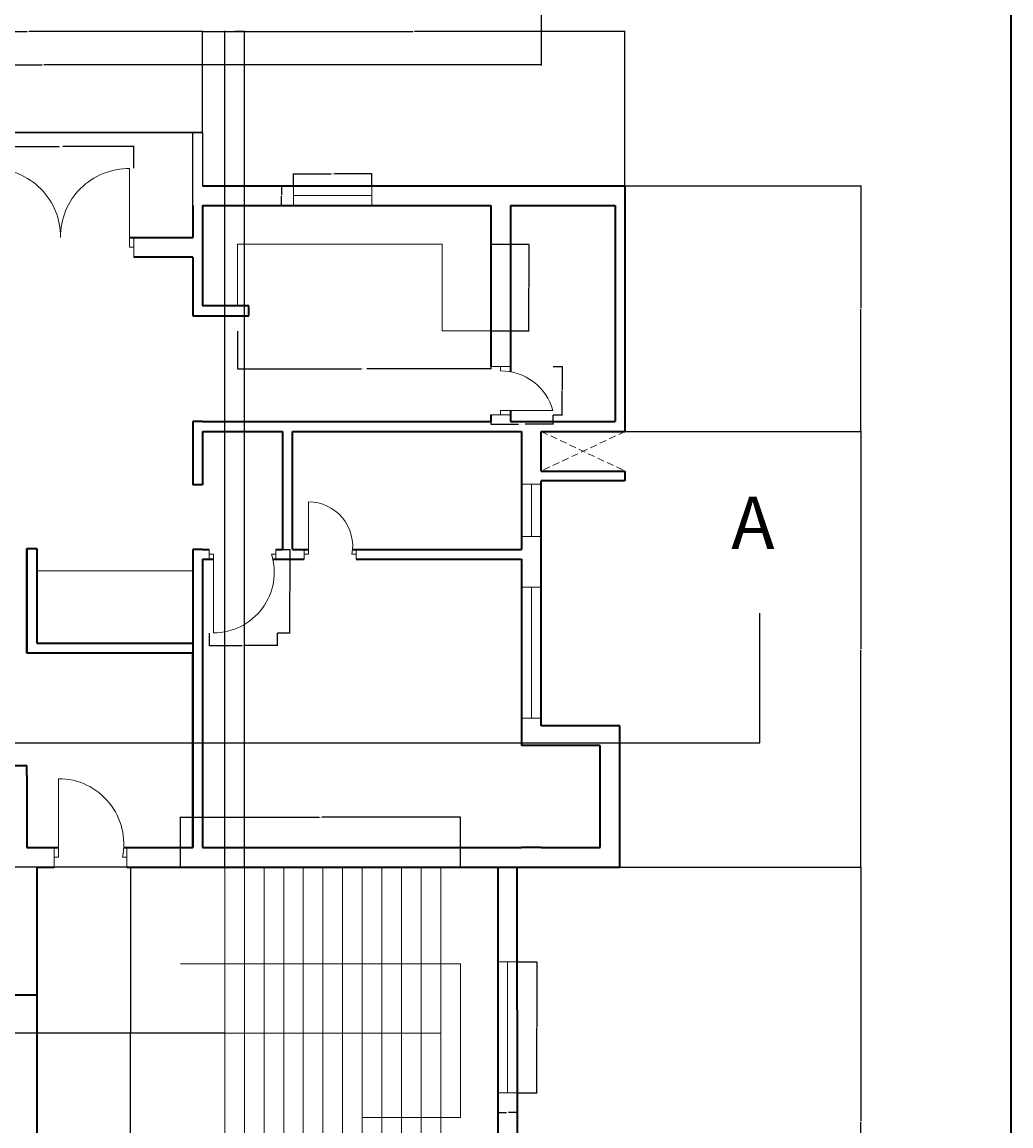
# Model space of a CAD drawing. Units: inches. Extents: x 2296 to 3812, y -1531 to 2564.
# Tile 9 of 10: x 3360 to 3812, y 1720 to 2226. Entities that reach past the tile are written whole.
import ezdxf

# ---------------------------------------------------------------- set-up
doc = ezdxf.new("R2010")
doc.units = ezdxf.units.IN
doc.linetypes.add('HIDDEN2', pattern=[4.7625, 3.175, -1.5875])
for name, color, linetype, lineweight in [('A-ANNO-DIMS', 2, 'Continuous', 18), ('A-ANNO-SYMB', 7, 'Continuous', 25), ('A-ANNO-TTLB', 7, 'Continuous', 35), ('A-DOOR', 3, 'Continuous', 18), ('A-FLOR-CASE', 8, 'Continuous', 18), ('A-FLOR-HRAL', 7, 'Continuous', 25), ('A-FLOR-STRS', 7, 'Continuous', 18), ('A-GLAZ', 4, 'Continuous', 18), ('A-WALL', 7, 'Continuous', 35), ('A-WALL-HIDN', 8, 'HIDDEN2', 18)]:
    doc.layers.add(name, color=color, linetype=linetype, lineweight=lineweight)
doc.styles.get("Standard").update_dxf_attribs({"font": 'arial.ttf'})
doc.dimstyles.get("Standard").update_dxf_attribs({"dimtxt": 0.18, "dimasz": 0.18, "dimexe": 0.18, "dimexo": 0.0625, "dimgap": 0.09, "dimtad": 0, "dimtih": 1, "dimtoh": 1, "dimdec": 4, "dimzin": 0, "dimdsep": 46, "dimtxsty": 'Standard', "dimcen": 0.09, "dimadec": 0, "dimazin": 0, "dimtfac": 1, "dimtdec": 4, "dimtofl": 0, "dimtmove": 0, "dimatfit": 3, "dimfxl": 1, "dimtolj": 1, "dimtzin": 0, "dimarcsym": 0})

# ---------------------------------------------------------------- blocks, each defined once
blk = doc.blocks.new('DOOR-SERVICE-24-NE')
for p, q in [((9, 22.16), (0, 22.16)), ((0, 22.16), (4.5, 22.16)), ((4.5, 22.16), (4.5, 20.16)), ((0, 0), (9, 0)), ((4.5, 0), (4.5, 2)), ((4.5, 2), (28.5, 2)), ((9, 0), (4.5, 0))]:
    blk.add_line(p, q)
blk.add_arc((4.5, -4.78), 24.94, 15.78, 90)
blk = doc.blocks.new('DOOR-BALCONY-PAIR-N')
for p, q in [((2, 4.5), (2, 40.5)), ((64.91, 4.5), (64.91, 40.5)), ((0, 9), (0, 0)), ((66.91, 9), (66.91, 0)), ((0, 0), (0, 4.5)), ((0, 4.5), (2, 4.5)), ((66.91, 4.5), (64.91, 4.5)), ((66.91, 0), (66.91, 4.5))]:
    blk.add_line(p, q)
for centre, radius, start, end in [((2, 9.22), 31.28, 359.5901, 90), ((64.41, 9.36), 31.14, 89.0831, 180.6679)]:
    blk.add_arc(centre, radius, start, end)
blk = doc.blocks.new('DOOR-BEDROOM-36-NE')
for p, q in [((0, 38.25), (0, 33.75)), ((0, 33.75), (0, 36)), ((0, 36), (0, 36)), ((0, 36), (2, 36)), ((2, 36), (2, 0)), ((30.56, 36), (28.56, 36)), ((30.56, 38.25), (30.56, 33.75)), ((30.56, 33.75), (30.56, 36))]:
    blk.add_line(p, q)
blk.add_arc((2, 27.8), 27.8, 270, 17.157)
blk = doc.blocks.new('DOOR-BATH-24-NE')
for p, q in [((2, 2.25), (2, 26.25)), ((0, 4.5), (0, 0)), ((0, 0), (0, 2.25)), ((0, 2.25), (2, 2.25)), ((23.89, 2.25), (21.89, 2.25)), ((23.89, 4.5), (23.89, 0)), ((23.89, 0), (23.89, 2.25))]:
    blk.add_line(p, q)
blk.add_arc((2, 6.01), 20.24, 349.2884, 90)
blk = doc.blocks.new('DOOR-ENTRY-36-N')
for p, q in [((2, 4.5), (2, 40.5)), ((0, 9), (0, 0)), ((33.22, 9), (33.22, 0)), ((0, 0), (0, 4.5)), ((0, 4.5), (2, 4.5)), ((33.22, 4.5), (31.22, 4.5)), ((33.22, 0), (33.22, 4.5))]:
    blk.add_line(p, q)
blk.add_arc((2, 10.64), 29.86, 348.1386, 90)
blk = doc.blocks.new('WIN-36-KITCHEN')
for p, q in [((0, 9), (0, 0)), ((36, 4.5), (36, 9)), ((36, 9), (36, 0)), ((0, 0), (0, 4.5)), ((0, 4.5), (36, 4.5))]:
    blk.add_line(p, q)
blk = doc.blocks.new('WIN-24-BATH')
for p, q in [((4.5, 24), (0, 24)), ((0, 24), (9, 24)), ((4.5, 0), (4.5, 24)), ((0, 0), (9, 0)), ((9, 0), (4.5, 0))]:
    blk.add_line(p, q)
blk = doc.blocks.new('WIN-60-JAMB-A')
for p, q in [((0, 60), (9, 60)), ((9, 60), (4.5, 60)), ((4.5, 60), (4.5, 0)), ((9, 0), (0, 0)), ((4.5, 0), (9, 0))]:
    blk.add_line(p, q)
blk = doc.blocks.new('WIN-60-STAIR')
for p, q in [((0, 59.99), (8.73, 60.01)), ((8.73, 60.01), (4.36, 60)), ((4.36, 60), (4.36, 0)), ((0, 0), (8.81, 0.01)), ((4.36, 0), (0, 0))]:
    blk.add_line(p, q)
blk = doc.blocks.new('STAIR-DOGLEG')
for p, q in [((20.27, 0), (20.27, 152.06)), ((29.27, 0), (29.27, 152.06)), ((38.27, 0), (38.27, 152.06)), ((47.27, 0), (47.27, 152.06)), ((56.27, 0), (56.27, 152.06)), ((65.27, 0), (65.27, 152.06)), ((74.27, 0), (74.27, 152.06)), ((83.27, 0), (83.27, 152.06)), ((92.27, 0), (92.27, 152.06)), ((101.27, 0), (101.27, 152.06)), ((110.27, 0), (110.27, 152.06)), ((119.27, 0), (119.27, 152.06)), ((0, 107.85), (128.27, 107.85)), ((128.27, 107.85), (128.27, 37.4)), ((20.27, 76.03), (119.27, 76.03)), ((128.27, 37.4), (83.27, 37.4))]:
    blk.add_line(p, q)
blk = doc.blocks.new('COUNTER-KITCHEN-N')
for p, q in [((0, 11.4), (0, 39.66)), ((0, 39.66), (93.66, 39.66)), ((93.66, 39.66), (93.66, 0)), ((93.66, 0), (115.91, 0))]:
    blk.add_line(p, q)
blk = doc.blocks.new('*D49')
at = {"layer": 'A-ANNO-DIMS', "color": 0, "lineweight": -2, "transparency": 16777216}
for p, q in [((3431.99, 1838.66), (3409.07, 1838.66)), ((3409.25, 1838.48), (3409.25, 1762.81)), ((3409.25, 1686.78), (3409.25, 1762.45)), ((3431.99, 1686.6), (3409.07, 1686.6))]:
    blk.add_line(p, q, dxfattribs=at)
at = {"layer": 'A-ANNO-DIMS', "color": 0, "transparency": 16777216}
for points in [[(3409.22, 1838.48), (3409.28, 1838.48), (3409.25, 1838.66)], [(3409.22, 1686.78), (3409.28, 1686.78), (3409.25, 1686.6)]]:
    blk.add_solid(points, dxfattribs=at)
at = {"layer": 'Defpoints', "color": 0, "transparency": 16777216}
for p in [(3409.25, 1838.66), (3432.06, 1838.66), (3432.06, 1686.6)]:
    blk.add_point(p, dxfattribs=at)
at = {"layer": 'A-ANNO-DIMS', "color": 0, "transparency": 16777216, "insert": (3409.25, 1762.63), "char_height": 0.18, "attachment_point": 5}
blk.add_mtext('\\A1;STAIR 152 TYP.', dxfattribs=at)
blk = doc.blocks.new('*D50')
at = {"layer": 'A-ANNO-DIMS', "color": 0, "lineweight": -2, "transparency": 16777216}
for p, q in [((3432.06, 1838.72), (3432.06, 1861.65)), ((3432.24, 1861.47), (3495.6, 1861.47)), ((3560.15, 1861.47), (3496.78, 1861.47)), ((3560.33, 1838.72), (3560.33, 1861.65))]:
    blk.add_line(p, q, dxfattribs=at)
at = {"layer": 'A-ANNO-DIMS', "color": 0, "transparency": 16777216}
for points in [[(3432.24, 1861.5), (3432.24, 1861.44), (3432.06, 1861.47)], [(3560.15, 1861.5), (3560.15, 1861.44), (3560.33, 1861.47)]]:
    blk.add_solid(points, dxfattribs=at)
at = {"layer": 'Defpoints', "color": 0, "transparency": 16777216}
for p in [(3560.33, 1861.47), (3432.06, 1838.66), (3560.33, 1838.66)]:
    blk.add_point(p, dxfattribs=at)
at = {"layer": 'A-ANNO-DIMS', "color": 0, "transparency": 16777216, "insert": (3496.19, 1861.47), "char_height": 0.18, "attachment_point": 5}
blk.add_mtext('\\A1;128 TYP.', dxfattribs=at)
blk = doc.blocks.new('*D53')
at = {"layer": 'A-ANNO-DIMS', "color": 0, "lineweight": -2, "transparency": 16777216}
for p, q in [((3458.25, 2084.15), (3458.25, 2066.64)), ((3574.16, 2084.15), (3574.16, 2066.64)), ((3458.43, 2066.82), (3514.95, 2066.82)), ((3573.98, 2066.82), (3517.46, 2066.82))]:
    blk.add_line(p, q, dxfattribs=at)
at = {"layer": 'A-ANNO-DIMS', "color": 0, "transparency": 16777216}
for points in [[(3458.43, 2066.85), (3458.43, 2066.79), (3458.25, 2066.82)], [(3573.98, 2066.85), (3573.98, 2066.79), (3574.16, 2066.82)]]:
    blk.add_solid(points, dxfattribs=at)
at = {"layer": 'Defpoints', "color": 0, "transparency": 16777216}
for p in [(3458.25, 2084.21), (3574.16, 2084.21), (3574.16, 2066.82)]:
    blk.add_point(p, dxfattribs=at)
at = {"layer": 'A-ANNO-DIMS', "color": 0, "transparency": 16777216, "insert": (3516.2, 2066.82), "char_height": 0.18, "attachment_point": 5}
blk.add_mtext('\\A1;COUNTER 116 TYP.', dxfattribs=at)
blk = doc.blocks.new('*D54')
at = {"layer": 'A-ANNO-DIMS', "color": 0, "lineweight": -2, "transparency": 16777216}
for p, q in [((3574.22, 2123.87), (3591.73, 2123.87)), ((3591.55, 2123.69), (3591.55, 2104.22)), ((3591.55, 2084.39), (3591.55, 2103.86)), ((3574.22, 2084.21), (3591.73, 2084.21))]:
    blk.add_line(p, q, dxfattribs=at)
at = {"layer": 'A-ANNO-DIMS', "color": 0, "transparency": 16777216}
for points in [[(3591.52, 2123.69), (3591.58, 2123.69), (3591.55, 2123.87)], [(3591.52, 2084.39), (3591.58, 2084.39), (3591.55, 2084.21)]]:
    blk.add_solid(points, dxfattribs=at)
at = {"layer": 'Defpoints', "color": 0, "transparency": 16777216}
for p in [(3574.16, 2123.87), (3591.55, 2123.87), (3574.16, 2084.21)]:
    blk.add_point(p, dxfattribs=at)
at = {"layer": 'A-ANNO-DIMS', "color": 0, "transparency": 16777216, "insert": (3591.55, 2104.04), "char_height": 0.18, "attachment_point": 5}
blk.add_mtext('\\A1;40 TYP.', dxfattribs=at)
blk = doc.blocks.new('*D61')
at = {"layer": 'A-ANNO-DIMS', "color": 0, "lineweight": -2, "transparency": 16777216}
for p, q in [((3574.16, 2045.69), (3574.16, 2041.3)), ((3602.66, 2045.69), (3602.66, 2041.3)), ((3574.34, 2041.48), (3586.88, 2041.48)), ((3602.48, 2041.48), (3589.94, 2041.48))]:
    blk.add_line(p, q, dxfattribs=at)
at = {"layer": 'A-ANNO-DIMS', "color": 0, "transparency": 16777216}
for points in [[(3574.34, 2041.51), (3574.34, 2041.45), (3574.16, 2041.48)], [(3602.48, 2041.51), (3602.48, 2041.45), (3602.66, 2041.48)]]:
    blk.add_solid(points, dxfattribs=at)
at = {"layer": 'Defpoints', "color": 0, "transparency": 16777216}
for p in [(3574.16, 2045.75), (3602.66, 2045.75), (3602.66, 2041.48)]:
    blk.add_point(p, dxfattribs=at)
at = {"layer": 'A-ANNO-DIMS', "color": 0, "transparency": 16777216, "insert": (3588.41, 2041.48), "char_height": 0.18, "attachment_point": 5}
blk.add_mtext('\\A1;SERVICE DOOR 29 TYP.', dxfattribs=at)
blk = doc.blocks.new('*D62')
at = {"layer": 'A-ANNO-DIMS', "color": 0, "lineweight": -2, "transparency": 16777216}
for p, q in [((3602.72, 2067.91), (3607.11, 2067.91)), ((3606.93, 2067.73), (3606.93, 2057.01)), ((3606.93, 2045.93), (3606.93, 2056.65)), ((3602.72, 2045.75), (3607.11, 2045.75))]:
    blk.add_line(p, q, dxfattribs=at)
at = {"layer": 'A-ANNO-DIMS', "color": 0, "transparency": 16777216}
for points in [[(3606.9, 2067.73), (3606.96, 2067.73), (3606.93, 2067.91)], [(3606.9, 2045.93), (3606.96, 2045.93), (3606.93, 2045.75)]]:
    blk.add_solid(points, dxfattribs=at)
at = {"layer": 'Defpoints', "color": 0, "transparency": 16777216}
for p in [(3602.66, 2067.91), (3606.93, 2067.91), (3602.66, 2045.75)]:
    blk.add_point(p, dxfattribs=at)
at = {"layer": 'A-ANNO-DIMS', "color": 0, "transparency": 16777216, "insert": (3606.93, 2056.83), "char_height": 0.18, "attachment_point": 5}
blk.add_mtext('\\A1;22 TYP.', dxfattribs=at)
blk = doc.blocks.new('*D63')
at = {"layer": 'A-ANNO-DIMS', "color": 0, "lineweight": -2, "transparency": 16777216}
for p, q in [((3343.86, 2158.72), (3343.86, 2168.88)), ((3344.04, 2168.7), (3376.46, 2168.7)), ((3410.59, 2168.7), (3378.17, 2168.7)), ((3410.77, 2158.72), (3410.77, 2168.88))]:
    blk.add_line(p, q, dxfattribs=at)
at = {"layer": 'A-ANNO-DIMS', "color": 0, "transparency": 16777216}
for points in [[(3344.04, 2168.73), (3344.04, 2168.67), (3343.86, 2168.7)], [(3410.59, 2168.73), (3410.59, 2168.67), (3410.77, 2168.7)]]:
    blk.add_solid(points, dxfattribs=at)
at = {"layer": 'Defpoints', "color": 0, "transparency": 16777216}
for p in [(3410.77, 2168.7), (3343.86, 2158.66), (3410.77, 2158.66)]:
    blk.add_point(p, dxfattribs=at)
at = {"layer": 'A-ANNO-DIMS', "color": 0, "transparency": 16777216, "insert": (3377.32, 2168.7), "char_height": 0.18, "attachment_point": 5}
blk.add_mtext('\\A1;PAIR 67 TYP.', dxfattribs=at)
blk = doc.blocks.new('*D65')
at = {"layer": 'A-ANNO-DIMS', "color": 0, "lineweight": -2, "transparency": 16777216}
for p, q in [((3476.44, 1984.16), (3482.29, 1984.16)), ((3482.11, 1983.98), (3482.11, 1965.22)), ((3482.11, 1946.09), (3482.11, 1964.85)), ((3476.44, 1945.91), (3482.29, 1945.91))]:
    blk.add_line(p, q, dxfattribs=at)
at = {"layer": 'A-ANNO-DIMS', "color": 0, "transparency": 16777216}
for points in [[(3482.08, 1983.98), (3482.14, 1983.98), (3482.11, 1984.16)], [(3482.08, 1946.09), (3482.14, 1946.09), (3482.11, 1945.91)]]:
    blk.add_solid(points, dxfattribs=at)
at = {"layer": 'Defpoints', "color": 0, "transparency": 16777216}
for p in [(3476.37, 1984.16), (3482.11, 1984.16), (3476.37, 1945.91)]:
    blk.add_point(p, dxfattribs=at)
at = {"layer": 'A-ANNO-DIMS', "color": 0, "transparency": 16777216, "insert": (3482.11, 1965.03), "char_height": 0.18, "attachment_point": 5}
blk.add_mtext('\\A1;DOOR 38 TYP.', dxfattribs=at)
blk = doc.blocks.new('*D66')
at = {"layer": 'A-ANNO-DIMS', "color": 0, "lineweight": -2, "transparency": 16777216}
for p, q in [((3445.21, 1945.85), (3445.21, 1939.99)), ((3476.37, 1945.85), (3476.37, 1939.99)), ((3445.39, 1940.17), (3460.26, 1940.17)), ((3476.19, 1940.17), (3461.32, 1940.17))]:
    blk.add_line(p, q, dxfattribs=at)
at = {"layer": 'A-ANNO-DIMS', "color": 0, "transparency": 16777216}
for points in [[(3445.39, 1940.2), (3445.39, 1940.14), (3445.21, 1940.17)], [(3476.19, 1940.2), (3476.19, 1940.14), (3476.37, 1940.17)]]:
    blk.add_solid(points, dxfattribs=at)
at = {"layer": 'Defpoints', "color": 0, "transparency": 16777216}
for p in [(3445.21, 1945.91), (3476.37, 1945.91), (3476.37, 1940.17)]:
    blk.add_point(p, dxfattribs=at)
at = {"layer": 'A-ANNO-DIMS', "color": 0, "transparency": 16777216, "insert": (3460.79, 1940.17), "char_height": 0.18, "attachment_point": 5}
blk.add_mtext('\\A1;31 TYP.', dxfattribs=at)
blk = doc.blocks.new('*D99')
at = {"layer": 'A-ANNO-DIMS', "color": 0, "lineweight": -2, "transparency": 16777216}
for p, q in [((3483.78, 2150.72), (3483.78, 2156.24)), ((3483.96, 2156.06), (3500.94, 2156.06)), ((3519.6, 2156.06), (3502.63, 2156.06)), ((3519.78, 2150.72), (3519.78, 2156.24))]:
    blk.add_line(p, q, dxfattribs=at)
at = {"layer": 'A-ANNO-DIMS', "color": 0, "transparency": 16777216}
for points in [[(3483.96, 2156.09), (3483.96, 2156.03), (3483.78, 2156.06)], [(3519.6, 2156.09), (3519.6, 2156.03), (3519.78, 2156.06)]]:
    blk.add_solid(points, dxfattribs=at)
at = {"layer": 'Defpoints', "color": 0, "transparency": 16777216}
for p in [(3519.78, 2156.06), (3483.78, 2150.66), (3519.78, 2150.66)]:
    blk.add_point(p, dxfattribs=at)
at = {"layer": 'A-ANNO-DIMS', "color": 0, "transparency": 16777216, "insert": (3501.78, 2156.06), "char_height": 0.18, "attachment_point": 5}
blk.add_mtext('\\A1;WIN. 36 TYP.', dxfattribs=at)
blk = doc.blocks.new('*D100')
at = {"layer": 'A-ANNO-DIMS', "color": 0, "lineweight": -2, "transparency": 16777216}
for p, q in [((3483.72, 2150.66), (3478.2, 2150.66)), ((3478.38, 2150.48), (3478.38, 2146.34)), ((3478.38, 2141.84), (3478.38, 2145.98)), ((3483.72, 2141.66), (3478.2, 2141.66))]:
    blk.add_line(p, q, dxfattribs=at)
at = {"layer": 'A-ANNO-DIMS', "color": 0, "transparency": 16777216}
for points in [[(3478.35, 2150.48), (3478.41, 2150.48), (3478.38, 2150.66)], [(3478.35, 2141.84), (3478.41, 2141.84), (3478.38, 2141.66)]]:
    blk.add_solid(points, dxfattribs=at)
at = {"layer": 'Defpoints', "color": 0, "transparency": 16777216}
for p in [(3478.38, 2150.66), (3483.78, 2150.66), (3483.78, 2141.66)]:
    blk.add_point(p, dxfattribs=at)
at = {"layer": 'A-ANNO-DIMS', "color": 0, "transparency": 16777216, "insert": (3478.38, 2146.16), "char_height": 0.18, "attachment_point": 5}
blk.add_mtext('\\A1;9 TYP.', dxfattribs=at)
blk = doc.blocks.new('*D113')
at = {"layer": 'A-ANNO-DIMS', "color": 0, "lineweight": -2, "transparency": 16777216}
for p, q in [((3586.37, 1795.35), (3595.49, 1795.35)), ((3595.31, 1795.17), (3595.31, 1765.53)), ((3595.31, 1735.52), (3595.31, 1765.16)), ((3586.37, 1735.34), (3595.49, 1735.34))]:
    blk.add_line(p, q, dxfattribs=at)
at = {"layer": 'A-ANNO-DIMS', "color": 0, "transparency": 16777216}
for points in [[(3595.28, 1795.17), (3595.34, 1795.17), (3595.31, 1795.35)], [(3595.28, 1735.52), (3595.34, 1735.52), (3595.31, 1735.34)]]:
    blk.add_solid(points, dxfattribs=at)
at = {"layer": 'Defpoints', "color": 0, "transparency": 16777216}
for p in [(3586.31, 1795.35), (3595.31, 1795.35), (3586.31, 1735.34)]:
    blk.add_point(p, dxfattribs=at)
at = {"layer": 'A-ANNO-DIMS', "color": 0, "transparency": 16777216, "insert": (3595.31, 1765.34), "char_height": 0.18, "attachment_point": 5}
blk.add_mtext('\\A1;WINDOW 60 TYP.', dxfattribs=at)
blk = doc.blocks.new('*D114')
at = {"layer": 'A-ANNO-DIMS', "color": 0, "lineweight": -2, "transparency": 16777216}
for p, q in [((3577.49, 1735.28), (3577.49, 1726.16)), ((3586.31, 1735.28), (3586.31, 1726.16)), ((3577.67, 1726.34), (3581.44, 1726.34)), ((3586.13, 1726.34), (3582.36, 1726.34))]:
    blk.add_line(p, q, dxfattribs=at)
at = {"layer": 'A-ANNO-DIMS', "color": 0, "transparency": 16777216}
for points in [[(3577.67, 1726.37), (3577.67, 1726.31), (3577.49, 1726.34)], [(3586.13, 1726.37), (3586.13, 1726.31), (3586.31, 1726.34)]]:
    blk.add_solid(points, dxfattribs=at)
at = {"layer": 'Defpoints', "color": 0, "transparency": 16777216}
for p in [(3577.49, 1735.34), (3586.31, 1735.34), (3586.31, 1726.34)]:
    blk.add_point(p, dxfattribs=at)
at = {"layer": 'A-ANNO-DIMS', "color": 0, "transparency": 16777216, "insert": (3581.9, 1726.34), "char_height": 0.18, "attachment_point": 5}
blk.add_mtext('\\A1;9 TYP.', dxfattribs=at)
blk = doc.blocks.new('*D132')
at = {"layer": 'A-ANNO-DIMS', "color": 0, "lineweight": -2, "transparency": 16777216}
for p, q in [((3282.51, 2175.09), (3282.51, 2221.56)), ((3282.69, 2221.38), (3361.88, 2221.38)), ((3441.98, 2221.38), (3362.79, 2221.38)), ((3442.16, 2175.09), (3442.16, 2221.56))]:
    blk.add_line(p, q, dxfattribs=at)
at = {"layer": 'A-ANNO-DIMS', "color": 0, "transparency": 16777216}
for points in [[(3282.69, 2221.41), (3282.69, 2221.35), (3282.51, 2221.38)], [(3441.98, 2221.41), (3441.98, 2221.35), (3442.16, 2221.38)]]:
    blk.add_solid(points, dxfattribs=at)
at = {"layer": 'Defpoints', "color": 0, "transparency": 16777216}
for p in [(3442.16, 2221.38), (3282.51, 2175.03), (3442.16, 2175.03)]:
    blk.add_point(p, dxfattribs=at)
at = {"layer": 'A-ANNO-DIMS', "color": 0, "transparency": 16777216, "insert": (3362.33, 2221.38), "char_height": 0.18, "attachment_point": 5}
blk.add_mtext('\\A1;159.65', dxfattribs=at)
blk = doc.blocks.new('*D133')
at = {"layer": 'A-ANNO-DIMS', "color": 0, "lineweight": -2, "transparency": 16777216}
for p, q in [((3442.16, 2175.09), (3442.16, 2221.56)), ((3442.34, 2221.38), (3538.52, 2221.38)), ((3635.48, 2221.38), (3539.29, 2221.38)), ((3635.66, 2150.72), (3635.66, 2221.56))]:
    blk.add_line(p, q, dxfattribs=at)
at = {"layer": 'A-ANNO-DIMS', "color": 0, "transparency": 16777216}
for points in [[(3442.34, 2221.41), (3442.34, 2221.35), (3442.16, 2221.38)], [(3635.48, 2221.41), (3635.48, 2221.35), (3635.66, 2221.38)]]:
    blk.add_solid(points, dxfattribs=at)
at = {"layer": 'Defpoints', "color": 0, "transparency": 16777216}
for p in [(3635.66, 2221.38), (3442.16, 2175.03), (3635.66, 2150.66)]:
    blk.add_point(p, dxfattribs=at)
at = {"layer": 'A-ANNO-DIMS', "color": 0, "transparency": 16777216, "insert": (3538.91, 2221.38), "char_height": 0.18, "attachment_point": 5}
blk.add_mtext('\\A1;193.5', dxfattribs=at)
blk = doc.blocks.new('*D136')
at = {"layer": 'A-ANNO-DIMS', "color": 0, "lineweight": -2, "transparency": 16777216}
for p, q in [((3633.38, 1838.66), (3743.91, 1838.66)), ((3743.73, 1838.48), (3743.73, 1722.31)), ((3743.73, 1605.78), (3743.73, 1721.95)), ((3642.06, 1605.6), (3743.91, 1605.6))]:
    blk.add_line(p, q, dxfattribs=at)
at = {"layer": 'A-ANNO-DIMS', "color": 0, "transparency": 16777216}
for points in [[(3743.7, 1838.48), (3743.76, 1838.48), (3743.73, 1838.66)], [(3743.7, 1605.78), (3743.76, 1605.78), (3743.73, 1605.6)]]:
    blk.add_solid(points, dxfattribs=at)
at = {"layer": 'Defpoints', "color": 0, "transparency": 16777216}
for p in [(3633.32, 1838.66), (3743.73, 1838.66), (3641.99, 1605.6)]:
    blk.add_point(p, dxfattribs=at)
at = {"layer": 'A-ANNO-DIMS', "color": 0, "transparency": 16777216, "insert": (3743.73, 1722.13), "char_height": 0.18, "attachment_point": 5}
blk.add_mtext('\\A1;233.06', dxfattribs=at)
blk = doc.blocks.new('*D137')
at = {"layer": 'A-ANNO-DIMS', "color": 0, "lineweight": -2, "transparency": 16777216}
for p, q in [((3635.72, 2038.16), (3743.91, 2038.16)), ((3743.73, 2037.98), (3743.73, 1938.59)), ((3743.73, 1838.84), (3743.73, 1938.23)), ((3633.38, 1838.66), (3743.91, 1838.66))]:
    blk.add_line(p, q, dxfattribs=at)
at = {"layer": 'A-ANNO-DIMS', "color": 0, "transparency": 16777216}
for points in [[(3743.7, 2037.98), (3743.76, 2037.98), (3743.73, 2038.16)], [(3743.7, 1838.84), (3743.76, 1838.84), (3743.73, 1838.66)]]:
    blk.add_solid(points, dxfattribs=at)
at = {"layer": 'Defpoints', "color": 0, "transparency": 16777216}
for p in [(3635.66, 2038.16), (3743.73, 2038.16), (3633.32, 1838.66)]:
    blk.add_point(p, dxfattribs=at)
at = {"layer": 'A-ANNO-DIMS', "color": 0, "transparency": 16777216, "insert": (3743.73, 1938.41), "char_height": 0.18, "attachment_point": 5}
blk.add_mtext('\\A1;199.5', dxfattribs=at)
blk = doc.blocks.new('*D138')
at = {"layer": 'A-ANNO-DIMS', "color": 0, "lineweight": -2, "transparency": 16777216}
for p, q in [((3635.72, 2150.66), (3743.91, 2150.66)), ((3743.73, 2150.48), (3743.73, 2094.59)), ((3743.73, 2038.34), (3743.73, 2094.23)), ((3635.72, 2038.16), (3743.91, 2038.16))]:
    blk.add_line(p, q, dxfattribs=at)
at = {"layer": 'A-ANNO-DIMS', "color": 0, "transparency": 16777216}
for points in [[(3743.7, 2150.48), (3743.76, 2150.48), (3743.73, 2150.66)], [(3743.7, 2038.34), (3743.76, 2038.34), (3743.73, 2038.16)]]:
    blk.add_solid(points, dxfattribs=at)
at = {"layer": 'Defpoints', "color": 0, "transparency": 16777216}
for p in [(3635.66, 2150.66), (3743.73, 2150.66), (3635.66, 2038.16)]:
    blk.add_point(p, dxfattribs=at)
at = {"layer": 'A-ANNO-DIMS', "color": 0, "transparency": 16777216, "insert": (3743.73, 2094.41), "char_height": 0.18, "attachment_point": 5}
blk.add_mtext('\\A1;112.5', dxfattribs=at)
blk = doc.blocks.new('*D140')
at = {"layer": 'A-ANNO-DIMS', "color": 0, "lineweight": -2, "transparency": 16777216}
for p, q in [((3452.33, 1838.72), (3452.33, 2221.56)), ((3452.51, 2221.38), (3456.68, 2221.38)), ((3461.15, 2221.38), (3456.98, 2221.38)), ((3461.33, 1838.72), (3461.33, 2221.56))]:
    blk.add_line(p, q, dxfattribs=at)
at = {"layer": 'A-ANNO-DIMS', "color": 0, "transparency": 16777216}
for points in [[(3452.51, 2221.41), (3452.51, 2221.35), (3452.33, 2221.38)], [(3461.15, 2221.41), (3461.15, 2221.35), (3461.33, 2221.38)]]:
    blk.add_solid(points, dxfattribs=at)
at = {"layer": 'Defpoints', "color": 0, "transparency": 16777216}
for p in [(3461.33, 2221.38), (3452.33, 1838.66), (3461.33, 1838.66)]:
    blk.add_point(p, dxfattribs=at)
at = {"layer": 'A-ANNO-DIMS', "color": 0, "transparency": 16777216, "insert": (3456.83, 2221.38), "char_height": 0.18, "attachment_point": 5}
blk.add_mtext('\\A1;9', dxfattribs=at)
blk = doc.blocks.new('*D141')
at = {"layer": 'A-ANNO-DIMS', "color": 0, "lineweight": -2, "transparency": 16777216}
for p, q in [((3452.27, 1838.66), (3014.48, 1838.66)), ((3014.66, 1838.48), (3014.66, 1800.83)), ((3014.66, 1762.81), (3014.66, 1800.46)), ((3452.27, 1762.63), (3014.48, 1762.63))]:
    blk.add_line(p, q, dxfattribs=at)
at = {"layer": 'A-ANNO-DIMS', "color": 0, "transparency": 16777216}
for points in [[(3014.63, 1838.48), (3014.69, 1838.48), (3014.66, 1838.66)], [(3014.63, 1762.81), (3014.69, 1762.81), (3014.66, 1762.63)]]:
    blk.add_solid(points, dxfattribs=at)
at = {"layer": 'Defpoints', "color": 0, "transparency": 16777216}
for p in [(3014.66, 1838.66), (3452.33, 1838.66), (3452.33, 1762.63)]:
    blk.add_point(p, dxfattribs=at)
at = {"layer": 'A-ANNO-DIMS', "color": 0, "transparency": 16777216, "insert": (3014.66, 1800.64), "char_height": 0.18, "attachment_point": 5}
blk.add_mtext('\\A1;76.03', dxfattribs=at)
blk = doc.blocks.new('*D159')
at = {"layer": 'A-ANNO-DIMS', "color": 0, "lineweight": -2, "transparency": 16777216}
for p, q in [((3140.84, 2277.72), (3140.84, 2205.81)), ((3597.32, 2277.72), (3597.32, 2205.81)), ((3141.02, 2205.99), (3368.68, 2205.99)), ((3597.14, 2205.99), (3369.48, 2205.99))]:
    blk.add_line(p, q, dxfattribs=at)
at = {"layer": 'A-ANNO-DIMS', "color": 0, "transparency": 16777216}
for points in [[(3141.02, 2206.02), (3141.02, 2205.96), (3140.84, 2205.99)], [(3597.14, 2206.02), (3597.14, 2205.96), (3597.32, 2205.99)]]:
    blk.add_solid(points, dxfattribs=at)
at = {"layer": 'Defpoints', "color": 0, "transparency": 16777216}
for p in [(3140.84, 2277.78), (3597.32, 2277.78), (3597.32, 2205.99)]:
    blk.add_point(p, dxfattribs=at)
at = {"layer": 'A-ANNO-DIMS', "color": 0, "transparency": 16777216, "insert": (3369.08, 2205.99), "char_height": 0.18, "attachment_point": 5}
blk.add_mtext('\\A1;456.5', dxfattribs=at)

msp = doc.modelspace()

# ---------------------------------------------------------------- linework, layer by layer
at = {"layer": 'A-ANNO-SYMB'}
for p, q in [((3697.3821, 1895.5359), (3697.3821, 1954.9583)), ((3061.0144, 1895.5359), (3697.3821, 1895.5359))]:
    msp.add_line(p, q, dxfattribs=at)
at = {"layer": 'A-ANNO-TTLB'}
msp.add_lwpolyline([(2296.1257, 2564.2989), (3812.4193, 2564.2989), (3812.4193, 1124.0028), (2296.1257, 1124.0028)], close=True, dxfattribs=at)
at = {"layer": 'A-FLOR-CASE'}
msp.add_line((3437.6588, 1974.3293), (3366.2648, 1974.3293), dxfattribs=at)
at = {"layer": 'A-FLOR-HRAL'}
for p, q in [((3442.1588, 2175.0276), (3308.6588, 2175.0276)), ((3313.1588, 2175.0276), (3442.1588, 2175.0276)), ((3437.6588, 2141.6578), (3437.6588, 2175.0276)), ((3442.1588, 2175.0276), (3442.1588, 2150.6578))]:
    msp.add_line(p, q, dxfattribs=at)
at = {"layer": 'A-WALL'}
for p, q in [((3442.1588, 2150.6578), (3635.6588, 2150.6578)), ((3442.1588, 2150.6578), (3635.6588, 2150.6578)), ((3635.6588, 2150.6578), (3635.6588, 2038.1578)), ((3437.6588, 2141.6578), (3437.6588, 2127.0276)), ((3442.1588, 2141.6578), (3442.1588, 2095.613)), ((3442.1588, 2141.6578), (3574.1588, 2141.6578)), ((3574.1588, 2141.6578), (3574.1588, 2067.9121)), ((3583.1588, 2141.6578), (3583.1588, 2065.5027)), ((3583.1588, 2141.6578), (3631.1588, 2141.6578)), ((3631.1588, 2141.6578), (3631.1588, 2042.6578)), ((3408.7726, 2127.0276), (3437.6588, 2127.0276)), ((3437.6588, 2118.0276), (3410.7726, 2118.0276)), ((3437.6588, 2118.0276), (3437.6588, 2091.113)), ((3463.3407, 2095.613), (3442.1588, 2095.613)), ((3463.3407, 2091.113), (3463.3407, 2095.613)), ((3437.6588, 2091.113), (3463.3407, 2091.113)), ((3583.1588, 2047.7544), (3583.1588, 2042.6578)), ((3437.6588, 2042.6578), (3437.6588, 2013.7336)), ((3442.1588, 2042.6578), (3437.6588, 2042.6578)), ((3442.1588, 2042.6578), (3574.1588, 2042.6578)), ((3574.1588, 2045.7544), (3574.1588, 2042.6578)), ((3583.1588, 2042.6578), (3631.1588, 2042.6578)), ((3583.1588, 2042.6578), (3631.1588, 2042.6578)), ((3442.1588, 2038.1578), (3442.1588, 2013.7336)), ((3442.1588, 2038.1578), (3478.8177, 2038.1578)), ((3478.8177, 2038.1578), (3478.8177, 1984.1578)), ((3483.3177, 2038.1578), (3588.3177, 2038.1578)), ((3483.3177, 1984.1578), (3483.3177, 2038.1578)), ((3483.3177, 2038.1578), (3588.3177, 2038.1578)), ((3588.3177, 2038.1578), (3588.3177, 1984.1578)), ((3597.3177, 2038.1578), (3635.6588, 2038.1578)), ((3597.3177, 2020.0533), (3597.3177, 2038.1578)), ((3597.3177, 2020.0533), (3635.6588, 2020.0533)), ((3635.6588, 2020.0533), (3635.6588, 2015.5533)), ((3635.6588, 2020.0533), (3635.6588, 2015.5533)), ((3442.1588, 2013.7336), (3437.6588, 2013.7336)), ((3597.3177, 1990.1003), (3597.3177, 2015.5533)), ((3635.6588, 2015.5533), (3597.3177, 2015.5533)), ((3597.3177, 2011.1578), (3597.3177, 2011.1578)), ((3597.3177, 1984.1578), (3597.3177, 2006.6578)), ((3361.7648, 1984.5954), (3361.7648, 1936.6578)), ((3361.7648, 1936.6578), (3361.7648, 1984.5954)), ((3361.7648, 1984.5954), (3366.2648, 1984.5954)), ((3366.2648, 1984.5954), (3366.2648, 1941.1578)), ((3437.6588, 1984.1578), (3437.6588, 1847.6578)), ((3442.1588, 1984.1578), (3437.6588, 1984.1578)), ((3437.6588, 1984.1578), (3437.6588, 1979.704)), ((3442.1588, 1984.1578), (3445.2067, 1984.1578)), ((3475.769, 1984.1578), (3478.8177, 1984.1578)), ((3483.3177, 1984.1578), (3490.7043, 1984.1578)), ((3510.8861, 1984.1578), (3588.3177, 1984.1578)), ((3597.3177, 1903.3996), (3597.3177, 1984.1578)), ((3442.1588, 1979.6578), (3442.1588, 1847.6578)), ((3442.1588, 1979.6578), (3447.2067, 1979.6578)), ((3474.3618, 1979.6578), (3488.7043, 1979.6578)), ((3512.59, 1979.6578), (3588.3177, 1979.6578)), ((3588.3177, 1979.6578), (3588.3177, 1894.3996)), ((3366.2648, 1941.1578), (3437.6588, 1941.1578)), ((3437.6588, 1936.6578), (3361.7648, 1936.6578)), ((3437.6588, 1847.6578), (3437.6588, 1936.6578)), ((3633.3177, 1903.3996), (3597.3177, 1903.3996)), ((3633.3177, 1894.3996), (3633.3177, 1903.3996)), ((3597.3177, 1894.3996), (3588.3177, 1894.3996)), ((3624.3177, 1894.3996), (3597.3177, 1894.3996)), ((3624.3177, 1847.6578), (3624.3177, 1894.3996)), ((3633.3177, 1838.6578), (3633.3177, 1894.3996)), ((3277.1479, 1885.1578), (3361.7648, 1885.1578)), ((3361.7648, 1880.6578), (3361.7648, 1885.1578)), ((3361.7648, 1880.6578), (3361.7648, 1847.6578)), ((3361.7648, 1847.6578), (3366.2648, 1847.6578)), ((3366.2648, 1847.6578), (3376.2592, 1847.6578)), ((3366.2648, 1847.6578), (3376.2592, 1847.6578)), ((3406.0762, 1847.6578), (3437.6588, 1847.6578)), ((3406.0762, 1847.6578), (3437.6588, 1847.6578)), ((3442.1588, 1847.6578), (3588.3177, 1847.6578)), ((3442.1588, 1847.6578), (3588.3177, 1847.6578)), ((3597.3177, 1847.6578), (3588.3177, 1847.6578)), ((3597.3177, 1847.6578), (3612.3177, 1847.6578)), ((3612.3177, 1847.6578), (3624.3177, 1847.6578)), ((3366.2648, 1838.6578), (3374.2592, 1838.6578)), ((3366.2648, 1838.6578), (3366.2648, 1780.1578)), ((3366.2648, 1838.6578), (3366.2648, 1789.1578)), ((3407.4836, 1838.6578), (3442.1588, 1838.6578)), ((3442.1588, 1838.6578), (3597.3177, 1838.6578)), ((3442.1588, 1838.6578), (3586.1588, 1838.6578)), ((3577.4944, 1686.6012), (3577.4944, 1838.6578)), ((3586.1588, 1838.6578), (3586.4944, 1605.6012)), ((3588.3177, 1838.6578), (3597.3177, 1838.6578)), ((3597.3177, 1838.6578), (3624.3177, 1838.6578)), ((3624.3177, 1838.6578), (3633.3177, 1838.6578)), ((3291.4894, 1780.1578), (3366.2648, 1780.1578)), ((3366.2648, 1780.1578), (3366.2648, 1674.9485))]:
    msp.add_line(p, q, dxfattribs=at)
at = {"layer": 'A-WALL-HIDN'}
for p, q in [((3635.6588, 2038.1578), (3597.3177, 2020.0533)), ((3597.3177, 2038.1578), (3635.6588, 2020.0533)), ((3635.6588, 2020.0533), (3635.6588, 2020.0533))]:
    msp.add_line(p, q, dxfattribs=at)

# ---------------------------------------------------------------- block references
at = {"layer": 'A-DOOR'}
for name, p in [('DOOR-BALCONY-PAIR-N', (3343.8604, 2118.028)), ('DOOR-SERVICE-24-NE', (3574.1584, 2045.754)), ('DOOR-BATH-24-NE', (3488.7044, 1979.658)), ('DOOR-BEDROOM-36-NE', (3445.2064, 1945.908)), ('DOOR-ENTRY-36-N', (3374.2594, 1838.658))]:
    msp.add_blockref(name, p, dxfattribs=at)
at = {"layer": 'A-FLOR-CASE'}
msp.add_blockref('COUNTER-KITCHEN-N', (3458.2474, 2084.209), dxfattribs=at)
at = {"layer": 'A-FLOR-STRS'}
msp.add_blockref('STAIR-DOGLEG', (3432.0574, 1686.601), dxfattribs=at)
at = {"layer": 'A-GLAZ'}
for name, p in [('WIN-36-KITCHEN', (3483.7844, 2141.658)), ('WIN-24-BATH', (3588.3174, 1990.1)), ('WIN-60-JAMB-A', (3588.3174, 1906.83)), ('WIN-60-STAIR', (3577.4944, 1735.339))]:
    msp.add_blockref(name, p, dxfattribs=at)

# ---------------------------------------------------------------- texts
at = {"layer": 'A-ANNO-SYMB', "insert": (3684.287, 2008.2679), "char_height": 24, "attachment_point": 1}
msp.add_mtext_dynamic_manual_height_columns('A', width=30.195569, gutter_width=12.5, heights=[0], dxfattribs=at)

# ---------------------------------------------------------------- dimensions: what is measured, and where the dimension line sits
at = {"layer": 'A-ANNO-DIMS'}
for base, p1, p2, override, picture, middle in [((3597.3177, 2205.9928), (3140.8418, 2277.7848), (3597.3177, 2277.7848), {"dimdec": 1, "dimlfac": 1, "dimrnd": 0, "dimzin": 0, "dimdsep": 46, "dimlunit": 2}, '*D159', (3369.0797, 2205.9928)), ((3442.1588, 2221.3776), (3282.5073, 2175.0276), (3442.1588, 2175.0276), {"dimdec": 2, "dimlfac": 1, "dimrnd": 0, "dimzin": 0, "dimdsep": 46, "dimlunit": 2}, '*D132', (3362.333, 2221.3776)), ((3635.6588, 2221.3776), (3442.1588, 2175.0276), (3635.6588, 2150.6578), {"dimdec": 1, "dimlfac": 1, "dimrnd": 0, "dimzin": 0, "dimdsep": 46, "dimlunit": 2}, '*D133', (3538.9088, 2221.3776)), ((3461.3277, 2221.3776), (3452.3277, 1838.6578), (3461.3277, 1838.6578), {"dimdec": 0, "dimlfac": 1, "dimrnd": 0, "dimzin": 0, "dimdsep": 46, "dimlunit": 2}, '*D140', (3456.8277, 2221.3776))]:
    dim = msp.add_linear_dim(base=base, p1=p1, p2=p2, dimstyle='Standard', override=override, dxfattribs=at)
    dim.commit()
    dim.dimension.update_dxf_attribs({"geometry": picture, "text_midpoint": middle})
for base, p1, p2, text, picture, middle in [((3410.7726, 2168.699), (3343.86, 2158.6621), (3410.7726, 2158.6621), 'PAIR <> TYP.', '*D63', (3377.3163, 2168.699)), ((3519.7848, 2156.0578), (3483.7848, 2150.6578), (3519.7848, 2150.6578), 'WIN. <> TYP.', '*D99', (3501.7848, 2156.0578)), ((3574.1588, 2066.8223), (3458.2476, 2084.2089), (3574.1588, 2084.2089), 'COUNTER <> TYP.', '*D53', (3516.2032, 2066.8223)), ((3602.6587500884, 2041.4794307932), (3574.1587500884, 2045.7544307932), (3602.6587500884, 2045.7544307932), 'SERVICE DOOR <> TYP.', '*D61', (3588.4087500884, 2041.4794307932)), ((3476.3728, 1940.1703), (3445.2067, 1945.9078), (3476.3728, 1945.9078), '<> TYP.', '*D66', (3460.7898, 1940.1703)), ((3560.3312, 1861.4663), (3432.0574, 1838.6578), (3560.3312, 1838.6578), '<> TYP.', '*D50', (3496.1943, 1861.4663)), ((3586.3075, 1726.3384), (3577.4944, 1735.3394), (3586.3075, 1735.3394), '<> TYP.', '*D114', (3581.901, 1726.3384))]:
    dim = msp.add_linear_dim(base=base, p1=p1, p2=p2, text=text, dimstyle='Standard', override={"dimdec": 0, "dimlfac": 1, "dimrnd": 0, "dimzin": 0, "dimdsep": 46, "dimlunit": 2}, dxfattribs=at)
    dim.commit()
    dim.dimension.update_dxf_attribs({"geometry": picture, "text_midpoint": middle})
for base, p1, p2, text, picture, middle in [((3478.3848, 2150.6578), (3483.7848, 2141.6578), (3483.7848, 2150.6578), '<> TYP.', '*D100', (3478.3848, 2146.1578)), ((3591.5454, 2123.8701), (3574.1588, 2084.2089), (3574.1588, 2123.8701), '<> TYP.', '*D54', (3591.5454, 2104.0395)), ((3606.9338, 2067.9121), (3602.6588, 2045.7544), (3602.6588, 2067.9121), '<> TYP.', '*D62', (3606.9338, 2056.8333)), ((3482.1103, 1984.1578), (3476.3728, 1945.9078), (3476.3728, 1984.1578), 'DOOR <> TYP.', '*D65', (3482.1103, 1965.0328)), ((3409.2489, 1838.6578), (3432.0574, 1686.6012), (3432.0574, 1838.6578), 'STAIR <> TYP.', '*D49', (3409.2489, 1762.6295)), ((3595.3085, 1795.3456), (3586.3075, 1735.3394), (3586.3075, 1795.3456), 'WINDOW <> TYP.', '*D113', (3595.3085, 1765.3425))]:
    dim = msp.add_linear_dim(base=base, p1=p1, p2=p2, angle=90, text=text, dimstyle='Standard', override={"dimdec": 0, "dimlfac": 1, "dimrnd": 0, "dimzin": 0, "dimdsep": 46, "dimlunit": 2}, dxfattribs=at)
    dim.commit()
    dim.dimension.update_dxf_attribs({"geometry": picture, "text_midpoint": middle})
for base, p1, p2, override, picture, middle in [((3743.7321, 2150.6578), (3635.6588, 2038.1578), (3635.6588, 2150.6578), {"dimdec": 1, "dimlfac": 1, "dimrnd": 0, "dimzin": 0, "dimdsep": 46, "dimlunit": 2}, '*D138', (3743.7321, 2094.4078)), ((3743.7321, 2038.1578), (3633.3177, 1838.6578), (3635.6588, 2038.1578), {"dimdec": 1, "dimlfac": 1, "dimrnd": 0, "dimzin": 0, "dimdsep": 46, "dimlunit": 2}, '*D137', (3743.7321, 1938.4078)), ((3014.6644, 1838.6578), (3452.3277, 1762.6295), (3452.3277, 1838.6578), {"dimdec": 2, "dimlfac": 1, "dimrnd": 0, "dimzin": 0, "dimdsep": 46, "dimlunit": 2}, '*D141', (3014.6644, 1800.6437)), ((3743.7321, 1838.6578), (3641.9944, 1605.6012), (3633.3177, 1838.6578), {"dimdec": 2, "dimlfac": 1, "dimrnd": 0, "dimzin": 0, "dimdsep": 46, "dimlunit": 2}, '*D136', (3743.7321, 1722.1295))]:
    dim = msp.add_linear_dim(base=base, p1=p1, p2=p2, angle=90, dimstyle='Standard', override=override, dxfattribs=at)
    dim.commit()
    dim.dimension.update_dxf_attribs({"geometry": picture, "text_midpoint": middle})

doc.saveas('drawing.dxf')
